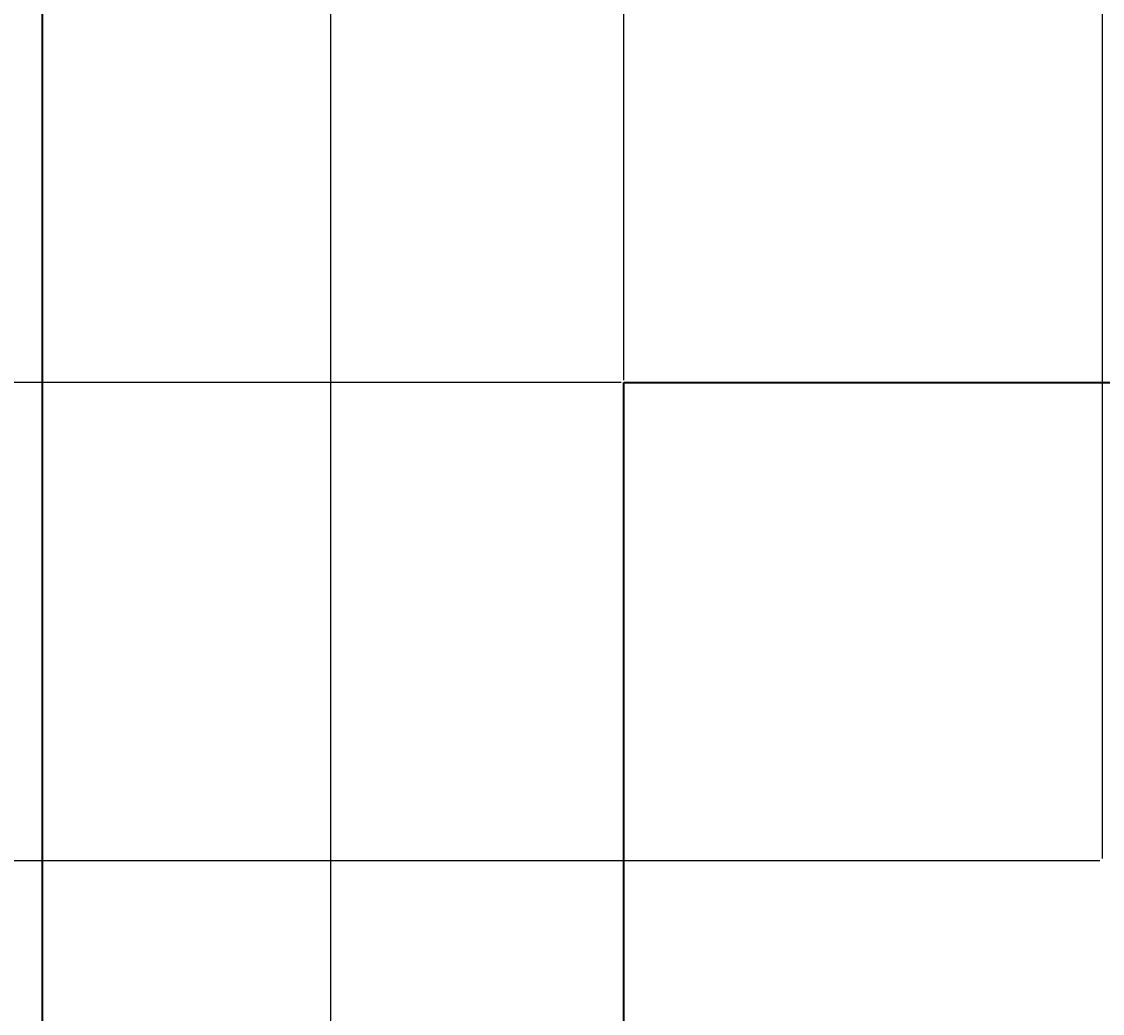
# Model space of a CAD drawing. Units: inches. Extents: x -6 to 289, y -8 to 323.
# Tile 45 of 107: x 19 to 46, y 273 to 298. Entities that reach past the tile are written whole.
import ezdxf

# ---------------------------------------------------------------- set-up
doc = ezdxf.new("R2010")
doc.units = ezdxf.units.IN
doc.header["$MEASUREMENT"] = 0
doc.layers.add('A-ANNO-DIMS', color=2, linetype='Continuous', lineweight=18)
doc.layers.add('A-ELEV', color=7, linetype='Continuous', lineweight=35)
doc.styles.get("Standard").update_dxf_attribs({"font": 'arial.ttf'})
doc.dimstyles.get("Standard").update_dxf_attribs({"dimtxt": 0.18, "dimasz": 0.18, "dimexe": 0.18, "dimexo": 0.0625, "dimgap": 0.09, "dimtad": 0, "dimtih": 1, "dimtoh": 1, "dimdec": 4, "dimzin": 0, "dimdsep": 46, "dimtxsty": 'Standard', "dimcen": 0.09, "dimadec": 0, "dimazin": 0, "dimtfac": 1, "dimtdec": 4, "dimtofl": 0, "dimtmove": 0, "dimatfit": 3, "dimfxl": 1, "dimtolj": 1, "dimtzin": 0, "dimarcsym": 0})

# ---------------------------------------------------------------- blocks, each defined once
blk = doc.blocks.new('*D5')
at = {"layer": 'A-ANNO-DIMS', "color": 0, "lineweight": -2, "transparency": 16777216}
for p, q in [((19.164, 307.351), (19.164, 322.969)), ((19.344, 322.789), (26.068, 322.789)), ((33.564, 322.789), (26.839, 322.789)), ((33.744, 289.105), (33.744, 322.969))]:
    blk.add_line(p, q, dxfattribs=at)
at = {"layer": 'A-ANNO-DIMS', "color": 0, "transparency": 16777216}
for points in [[(19.344, 322.819), (19.344, 322.759), (19.164, 322.789)], [(33.564, 322.819), (33.564, 322.759), (33.744, 322.789)]]:
    blk.add_solid(points, dxfattribs=at)
at = {"layer": 'Defpoints', "color": 0, "transparency": 16777216}
for p in [(33.744, 322.789), (19.164, 307.289), (33.744, 289.043)]:
    blk.add_point(p, dxfattribs=at)
at = {"layer": 'A-ANNO-DIMS', "color": 0, "transparency": 16777216, "insert": (26.454, 322.789), "char_height": 0.18, "attachment_point": 5}
blk.add_mtext('\\A1;14.58', dxfattribs=at)
blk = doc.blocks.new('*D6')
at = {"layer": 'A-ANNO-DIMS', "color": 0, "lineweight": -2, "transparency": 16777216}
for p, q in [((33.744, 289.105), (33.744, 322.969)), ((33.924, 322.789), (39.534, 322.789)), ((45.564, 322.789), (39.953, 322.789)), ((45.744, 277.105), (45.744, 322.969))]:
    blk.add_line(p, q, dxfattribs=at)
at = {"layer": 'A-ANNO-DIMS', "color": 0, "transparency": 16777216}
for points in [[(33.924, 322.819), (33.924, 322.759), (33.744, 322.789)], [(45.564, 322.819), (45.564, 322.759), (45.744, 322.789)]]:
    blk.add_solid(points, dxfattribs=at)
at = {"layer": 'Defpoints', "color": 0, "transparency": 16777216}
for p in [(45.744, 322.789), (33.744, 289.043), (45.744, 277.043)]:
    blk.add_point(p, dxfattribs=at)
at = {"layer": 'A-ANNO-DIMS', "color": 0, "transparency": 16777216, "insert": (39.744, 322.789), "char_height": 0.18, "attachment_point": 5}
blk.add_mtext('\\A1;12', dxfattribs=at)
blk = doc.blocks.new('*D7')
at = {"layer": 'A-ANNO-DIMS', "color": 0, "lineweight": -2, "transparency": 16777216}
for p, q in [((45.744, 277.105), (45.744, 322.969)), ((45.924, 322.789), (66.325, 322.789)), ((87.521, 322.789), (67.119, 322.789)), ((87.701, 277.105), (87.701, 322.969))]:
    blk.add_line(p, q, dxfattribs=at)
at = {"layer": 'A-ANNO-DIMS', "color": 0, "transparency": 16777216}
for points in [[(45.924, 322.819), (45.924, 322.759), (45.744, 322.789)], [(87.521, 322.819), (87.521, 322.759), (87.701, 322.789)]]:
    blk.add_solid(points, dxfattribs=at)
at = {"layer": 'Defpoints', "color": 0, "transparency": 16777216}
for p in [(87.701, 322.789), (45.744, 277.043), (87.701, 277.043)]:
    blk.add_point(p, dxfattribs=at)
at = {"layer": 'A-ANNO-DIMS', "color": 0, "transparency": 16777216, "insert": (66.722, 322.789), "char_height": 0.18, "attachment_point": 5}
blk.add_mtext('\\A1;41.96', dxfattribs=at)
blk = doc.blocks.new('*D19')
at = {"layer": 'A-ANNO-DIMS', "color": 0, "lineweight": -2, "transparency": 16777216}
for p, q in [((45.681, 277.043), (-5.737, 277.043)), ((-5.557, 276.863), (-5.557, 179.825)), ((-5.557, 82.423), (-5.557, 179.461)), ((45.681, 82.243), (-5.737, 82.243))]:
    blk.add_line(p, q, dxfattribs=at)
at = {"layer": 'A-ANNO-DIMS', "color": 0, "transparency": 16777216}
for points in [[(-5.587, 276.863), (-5.527, 276.863), (-5.557, 277.043)], [(-5.587, 82.423), (-5.527, 82.423), (-5.557, 82.243)]]:
    blk.add_solid(points, dxfattribs=at)
at = {"layer": 'Defpoints', "color": 0, "transparency": 16777216}
for p in [(-5.557, 277.043), (45.744, 277.043), (45.744, 82.243)]:
    blk.add_point(p, dxfattribs=at)
at = {"layer": 'A-ANNO-DIMS', "color": 0, "transparency": 16777216, "insert": (-5.557, 179.643), "char_height": 0.18, "attachment_point": 5}
blk.add_mtext('\\A1;194.8', dxfattribs=at)
blk = doc.blocks.new('*D20')
at = {"layer": 'A-ANNO-DIMS', "color": 0, "lineweight": -2, "transparency": 16777216}
for p, q in [((33.681, 289.043), (-5.737, 289.043)), ((-5.557, 288.863), (-5.557, 283.223)), ((-5.557, 277.223), (-5.557, 282.862)), ((45.681, 277.043), (-5.737, 277.043))]:
    blk.add_line(p, q, dxfattribs=at)
at = {"layer": 'A-ANNO-DIMS', "color": 0, "transparency": 16777216}
for points in [[(-5.587, 288.863), (-5.527, 288.863), (-5.557, 289.043)], [(-5.587, 277.223), (-5.527, 277.223), (-5.557, 277.043)]]:
    blk.add_solid(points, dxfattribs=at)
at = {"layer": 'Defpoints', "color": 0, "transparency": 16777216}
for p in [(-5.557, 289.043), (33.744, 289.043), (45.744, 277.043)]:
    blk.add_point(p, dxfattribs=at)
at = {"layer": 'A-ANNO-DIMS', "color": 0, "transparency": 16777216, "insert": (-5.557, 283.043), "char_height": 0.18, "attachment_point": 5}
blk.add_mtext('\\A1;12', dxfattribs=at)
blk = doc.blocks.new('*D21')
at = {"layer": 'A-ANNO-DIMS', "color": 0, "lineweight": -2, "transparency": 16777216}
for p, q in [((19.101, 307.289), (-5.737, 307.289)), ((-5.557, 307.109), (-5.557, 298.348)), ((-5.557, 289.223), (-5.557, 297.984)), ((33.681, 289.043), (-5.737, 289.043))]:
    blk.add_line(p, q, dxfattribs=at)
at = {"layer": 'A-ANNO-DIMS', "color": 0, "transparency": 16777216}
for points in [[(-5.587, 307.109), (-5.527, 307.109), (-5.557, 307.289)], [(-5.587, 289.223), (-5.527, 289.223), (-5.557, 289.043)]]:
    blk.add_solid(points, dxfattribs=at)
at = {"layer": 'Defpoints', "color": 0, "transparency": 16777216}
for p in [(-5.557, 307.289), (19.164, 307.289), (33.744, 289.043)]:
    blk.add_point(p, dxfattribs=at)
at = {"layer": 'A-ANNO-DIMS', "color": 0, "transparency": 16777216, "insert": (-5.557, 298.166), "char_height": 0.18, "attachment_point": 5}
blk.add_mtext('\\A1;18.246', dxfattribs=at)
blk = doc.blocks.new('*D22')
at = {"layer": 'A-ANNO-DIMS', "color": 0, "lineweight": -2, "transparency": 16777216}
for p, q in [((19.101, 307.289), (-5.737, 307.289)), ((-5.557, 307.109), (-5.557, 157.471)), ((-5.557, 7.469), (-5.557, 157.107)), ((11.907, 7.289), (-5.737, 7.289))]:
    blk.add_line(p, q, dxfattribs=at)
at = {"layer": 'A-ANNO-DIMS', "color": 0, "transparency": 16777216}
for points in [[(-5.587, 307.109), (-5.527, 307.109), (-5.557, 307.289)], [(-5.587, 7.469), (-5.527, 7.469), (-5.557, 7.289)]]:
    blk.add_solid(points, dxfattribs=at)
at = {"layer": 'Defpoints', "color": 0, "transparency": 16777216}
for p in [(19.164, 307.289), (-5.557, 7.289), (11.969, 7.289)]:
    blk.add_point(p, dxfattribs=at)
at = {"layer": 'A-ANNO-DIMS', "color": 0, "transparency": 16777216, "insert": (-5.557, 157.289), "char_height": 0.18, "attachment_point": 5}
blk.add_mtext('\\A1;300', dxfattribs=at)
blk = doc.blocks.new('*D27')
at = {"layer": 'A-ANNO-DIMS', "color": 0, "lineweight": -2, "transparency": 16777216}
for p, q in [((19.226, 307.289), (288.653, 307.289)), ((288.473, 307.109), (288.473, 277.471)), ((288.473, 247.469), (288.473, 277.107)), ((247.226, 247.289), (288.653, 247.289))]:
    blk.add_line(p, q, dxfattribs=at)
at = {"layer": 'A-ANNO-DIMS', "color": 0, "transparency": 16777216}
for points in [[(288.443, 307.109), (288.503, 307.109), (288.473, 307.289)], [(288.443, 247.469), (288.503, 247.469), (288.473, 247.289)]]:
    blk.add_solid(points, dxfattribs=at)
at = {"layer": 'Defpoints', "color": 0, "transparency": 16777216}
for p in [(19.164, 307.289), (288.473, 307.289), (247.164, 247.289)]:
    blk.add_point(p, dxfattribs=at)
at = {"layer": 'A-ANNO-DIMS', "color": 0, "transparency": 16777216, "insert": (288.473, 277.289), "char_height": 0.18, "attachment_point": 5}
blk.add_mtext('\\A1;60', dxfattribs=at)
blk = doc.blocks.new('*D57')
at = {"layer": 'A-ANNO-DIMS', "color": 0, "lineweight": -2, "transparency": 16777216}
for p, q in [((9.943, 68.495), (9.943, 322.969)), ((10.123, 322.789), (17.788, 322.789)), ((26.223, 322.789), (18.558, 322.789)), ((26.403, 68.495), (26.403, 322.969))]:
    blk.add_line(p, q, dxfattribs=at)
at = {"layer": 'A-ANNO-DIMS', "color": 0, "transparency": 16777216}
for points in [[(10.123, 322.819), (10.123, 322.759), (9.943, 322.789)], [(26.223, 322.819), (26.223, 322.759), (26.403, 322.789)]]:
    blk.add_solid(points, dxfattribs=at)
at = {"layer": 'Defpoints', "color": 0, "transparency": 16777216}
for p in [(26.403, 322.789), (9.943, 68.432), (26.403, 68.432)]:
    blk.add_point(p, dxfattribs=at)
at = {"layer": 'A-ANNO-DIMS', "color": 0, "transparency": 16777216, "insert": (18.173, 322.789), "char_height": 0.18, "attachment_point": 5}
blk.add_mtext('\\A1;16.46', dxfattribs=at)

msp = doc.modelspace()

# ---------------------------------------------------------------- linework, layer by layer
at = {"layer": 'A-ELEV'}
msp.add_line((19.1638, 307.2888), (19.1638, 68.4322), dxfattribs=at)
msp.add_lwpolyline([(33.7437, 289.0427), (99.7007, 289.0427), (99.7007, 70.2425), (33.7437, 70.2425)], close=True, dxfattribs=at)

# ---------------------------------------------------------------- dimensions: what is measured, and where the dimension line sits
at = {"layer": 'A-ANNO-DIMS'}
for base, p1, p2, override, picture, middle in [((26.403, 322.7888), (9.943, 68.4322), (26.403, 68.4322), {"dimdec": 2, "dimlfac": 1, "dimrnd": 0, "dimzin": 0, "dimdsep": 46, "dimlunit": 2}, '*D57', (18.173, 322.7888)), ((33.7437, 322.7888), (19.1638, 307.2888), (33.7437, 289.0427), {"dimdec": 2, "dimlfac": 1, "dimrnd": 0, "dimzin": 0, "dimdsep": 46, "dimlunit": 2}, '*D5', (26.4537, 322.7888)), ((45.7437, 322.7888), (33.7437, 289.0427), (45.7437, 277.0427), {"dimdec": 0, "dimlfac": 1, "dimrnd": 0, "dimzin": 0, "dimdsep": 46, "dimlunit": 2}, '*D6', (39.7437, 322.7888)), ((87.7007, 322.7888), (45.7437, 277.0427), (87.7007, 277.0427), {"dimdec": 2, "dimlfac": 1, "dimrnd": 0, "dimzin": 0, "dimdsep": 46, "dimlunit": 2}, '*D7', (66.7222, 322.7888))]:
    dim = msp.add_linear_dim(base=base, p1=p1, p2=p2, dimstyle='Standard', override=override, dxfattribs=at)
    dim.commit()
    dim.dimension.update_dxf_attribs({"geometry": picture, "text_midpoint": middle})
for base, p1, p2, override, picture, middle in [((-5.557, 307.2888), (33.7437, 289.0427), (19.1638, 307.2888), {"dimdec": 3, "dimlfac": 1, "dimrnd": 0, "dimzin": 0, "dimdsep": 46, "dimlunit": 2}, '*D21', (-5.557, 298.1657)), ((-5.557, 7.2888), (19.1638, 307.2888), (11.9692, 7.2888), {"dimdec": 0, "dimlfac": 1, "dimrnd": 0, "dimzin": 0, "dimdsep": 46, "dimlunit": 2}, '*D22', (-5.557, 157.2888)), ((288.4733, 307.2888), (247.1638, 247.2888), (19.1638, 307.2888), {"dimdec": 0, "dimlfac": 1, "dimrnd": 0, "dimzin": 0, "dimdsep": 46, "dimlunit": 2}, '*D27', (288.4733, 277.2888)), ((-5.557, 289.0427), (45.7437, 277.0427), (33.7437, 289.0427), {"dimdec": 0, "dimlfac": 1, "dimrnd": 0, "dimzin": 0, "dimdsep": 46, "dimlunit": 2}, '*D20', (-5.557, 283.0427)), ((-5.557, 277.0427), (45.7437, 82.2425), (45.7437, 277.0427), {"dimdec": 1, "dimlfac": 1, "dimrnd": 0, "dimzin": 0, "dimdsep": 46, "dimlunit": 2}, '*D19', (-5.557, 179.6426))]:
    dim = msp.add_linear_dim(base=base, p1=p1, p2=p2, angle=90, dimstyle='Standard', override=override, dxfattribs=at)
    dim.commit()
    dim.dimension.update_dxf_attribs({"geometry": picture, "text_midpoint": middle})

doc.saveas('drawing.dxf')
